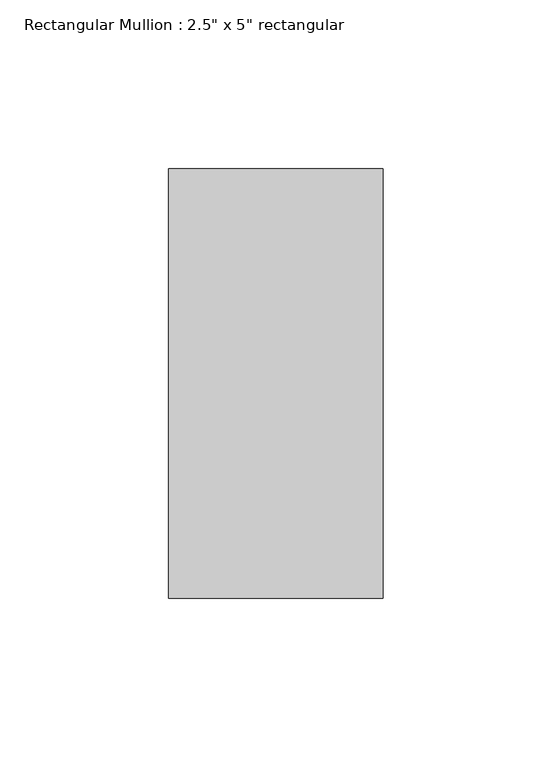
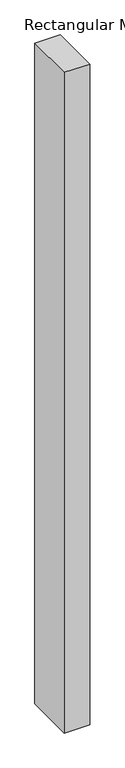
"""IFC4 building model written with IfcOpenShell, lengths in millimetres: member geometry."""

from ifc_helpers import new_model, si_unit, frame, origin, place, context, project, spatial, polyline, outline, extrude, source, transform, mapped, element, save


def member_183d059d(model_context):
    return source(origin(), model_context, "Body", "SweptSolid", [
        extrude(outline(polyline([(0.0, 63.5), (0.0, -63.5), (-63.5, -63.5), (-63.5, 63.5), (0.0, 63.5)])), frame((0.0, 0.0, -1747.5125275), z_axis=(0.0, 0.0, 1.0), x_axis=(1.0, 0.0, 0.0)), (0.0, 0.0, 1.0), 1747.5125275),
    ])


if __name__ == "__main__":
    model = new_model("IFC4")
    model_context = context("Model", 3, world=origin())
    ifc_project = project(units=[si_unit("LENGTHUNIT", "METRE", prefix="MILLI")], contexts=[model_context])
    site = spatial("IfcSite", under=ifc_project)
    building = spatial("IfcBuilding", under=site)
    placement = place(None, origin())
    member_shape = member_183d059d(model_context)
    element("IfcMember", 1, ObjectType="Rectangular Mullion : 2.5\" x 5\" rectangular", at=placement, inside=building, context=model_context, shape_type="MappedRepresentation", body=[
        mapped(member_shape, transform((0.0, 0.0, 0.0), x_axis=(1.0, 0.0, 0.0), y_axis=(0.0, 1.0, 0.0), z_axis=(0.0, 0.0, 1.0))),
    ])
    save(model, "model.ifc")

# Revit data of these elements
# Type "Rectangular Mullion : 2.5\" x 5\" rectangular"
#   built-in parameter 1007304 = 0.416667 (stored number, unit not read)
#   built-in parameter 1007301 = 0.104167 (stored number, unit not read)
#   built-in parameter 1007300 = 0.104167 (stored number, unit not read)
# Element 1 (IfcMember, "Rectangular Mullion : 2.5\" x 5\" rectangular")
#   Materials on its faces: "Aluminum"
# Materials
#   "Aluminum": class "Metal", colour RGB 247 247 247, transparency 0, Description = "Aluminum 6061", Cost = 0
